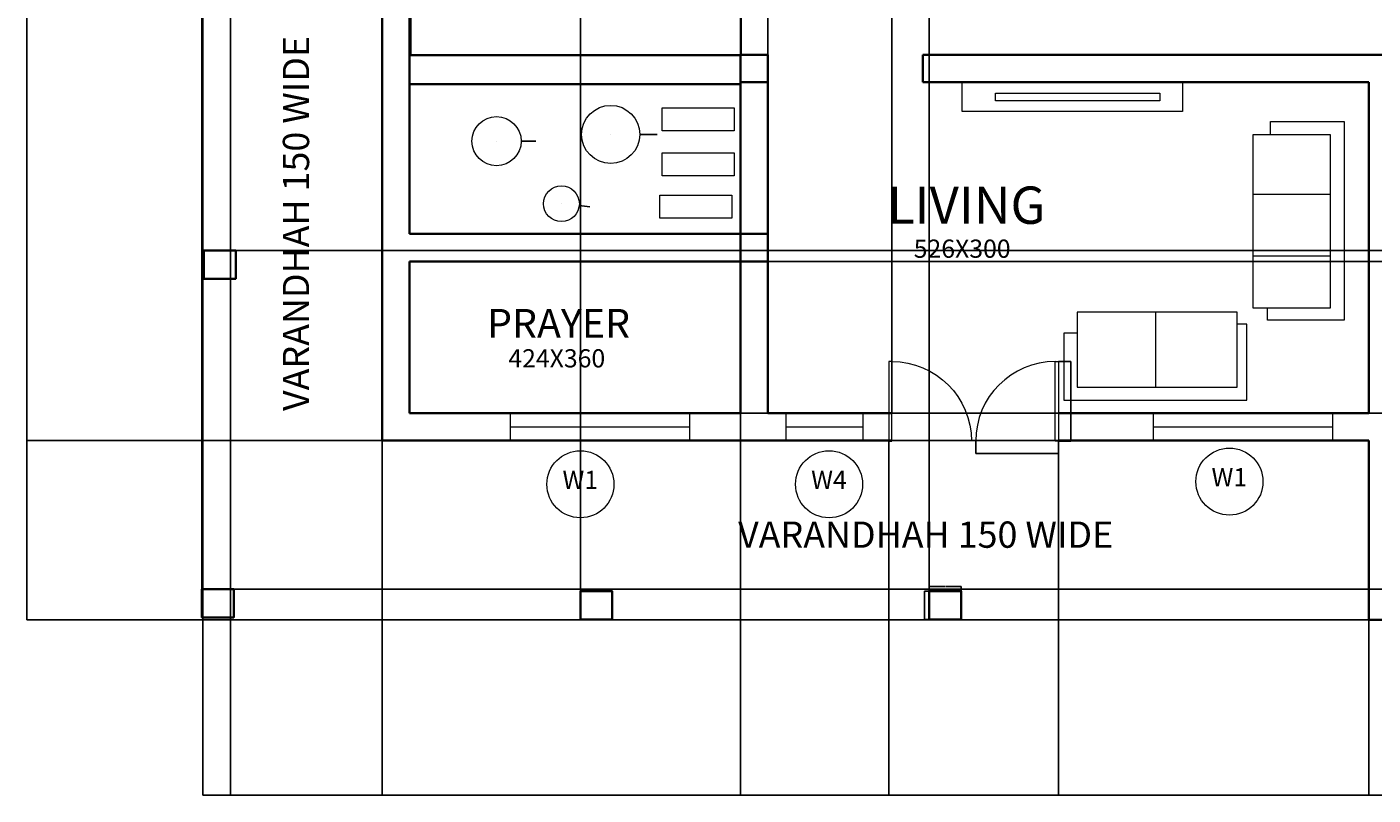
# Model space of a CAD drawing. Units: millimetres. Extents: x -2968 to 14333, y -2966 to 13411.
# Tile 1 of 3: x -2968 to 8301, y -2966 to 3466. Entities that reach past the tile are written whole.
import ezdxf

# ---------------------------------------------------------------- set-up
doc = ezdxf.new("R2010")
doc.units = ezdxf.units.MM
doc.header["$MEASUREMENT"] = 0
for name, color, linetype, lineweight in [('A-ANNO-DIMS', 2, 'Continuous', 18), ('A-ANNO-SYMB', 3, 'Continuous', 13), ('A-AREA-IDEN', 7, 'Continuous', 18), ('A-COLS', 7, 'Continuous', 35), ('A-DOOR', 3, 'Continuous', 18), ('A-FLOR-DETL', 8, 'Continuous', 18), ('A-FLOR-EDGE', 7, 'Continuous', 25), ('A-FURN', 8, 'Continuous', 18), ('A-GLAZ', 4, 'Continuous', 18), ('A-WALL', 7, 'Continuous', 35)]:
    doc.layers.add(name, color=color, linetype=linetype, lineweight=lineweight)
doc.styles.get("Standard").update_dxf_attribs({"font": 'arial.ttf'})
doc.dimstyles.get("Standard").update_dxf_attribs({"dimtxt": 0.18, "dimasz": 0.18, "dimexe": 0.18, "dimexo": 0.0625, "dimgap": 0.09, "dimtad": 0, "dimtih": 1, "dimtoh": 1, "dimdec": 4, "dimzin": 0, "dimdsep": 46, "dimtxsty": 'Standard', "dimcen": 0.09, "dimadec": 0, "dimazin": 0, "dimtfac": 1, "dimtdec": 4, "dimtofl": 0, "dimtmove": 0, "dimatfit": 3, "dimfxl": 1, "dimtolj": 1, "dimtzin": 0, "dimarcsym": 0})

# ---------------------------------------------------------------- blocks, each defined once
blk = doc.blocks.new('DOOR-SWING-666')
blk.add_lwpolyline([(666.2992070210612, -7.87249337009e-05), (666.2992070210612, 666.0645318323222), (692.9797223629398, 666.0645318323222), (692.9797223629398, -7.87249337009e-05)], close=True)
blk.add_arc((666.2992070210612, -7.87249337009e-05), 666.2995763929106, 90, 180)
blk = doc.blocks.new('WIN-1500')
for p, q in [((-0.0001454069465439, 230.0001364428754), (-0.0001454069465439, 0.0001364428753732)), ((1499.999854593053, 230.0001364428754), (1499.999854593053, 0.0001364428753732)), ((-0.0001454069465439, 115.0001364428753), (1499.999854593053, 115.0001364428753))]:
    blk.add_line(p, q)
blk = doc.blocks.new('WIN-645')
for p, q in [((-0.0001783325678844, 645.3165217330161), (229.9998216674321, 645.3165217330161)), ((114.9998216674321, 645.3165217330161), (114.9998216674321, 9.39247611313e-05)), ((-0.0001783325678844, 9.39247611313e-05), (229.9998216674321, 9.39247611313e-05))]:
    blk.add_line(p, q)
blk = doc.blocks.new('VERANDAH-POST')
blk.add_lwpolyline([(-5.84108229305e-05, 235.3216454025205), (266.2404368537072, 235.3216454025205), (266.2404368537072, -0.0003482651118247), (-5.84108229305e-05, -0.0003482651118247)], close=True)
blk = doc.blocks.new('TAG-W1')
blk.add_circle((280.793431040287, 280.7932079668344), 280.7929963504647)
blk.add_text('W1', height=152.3112078732942).set_placement((130.9915239926576, 241.6268535788358))
blk = doc.blocks.new('TAG-W4')
blk.add_circle((280.792632550478, 280.7926029835935), 280.7929963504647)
blk.add_text('W4', height=152.3112078732942).set_placement((130.9907255028486, 241.6262485955949))
blk = doc.blocks.new('*D26')
at = {"layer": 'A-ANNO-DIMS', "color": 0, "lineweight": -2, "transparency": 16777216}
for p, q in [((4974.697580339908, -2.140366612195065), (4974.697580339908, -106.2048803724133)), ((4974.877580339908, -106.0248803724133), (5319.720982278243, -106.0248803724133)), ((5667.497672074696, -106.0248803724133), (5322.654270136361, -106.0248803724133)), ((5667.677672074696, -2.140366612195065), (5667.677672074696, -106.2048803724133))]:
    blk.add_line(p, q, dxfattribs=at)
at = {"layer": 'A-ANNO-DIMS', "color": 0, "transparency": 16777216}
for points in [[(4974.877580339908, -105.9948803724133), (4974.877580339908, -106.0548803724133), (4974.697580339908, -106.0248803724133)], [(5667.497672074696, -105.9948803724133), (5667.497672074696, -106.0548803724133), (5667.677672074696, -106.0248803724133)]]:
    blk.add_solid(points, dxfattribs=at)
at = {"layer": 'Defpoints', "color": 0, "transparency": 16777216}
for p in [(4974.697580339908, -2.077866612195065), (5667.677672074696, -2.077866612195065), (5667.677672074696, -106.0248803724133)]:
    blk.add_point(p, dxfattribs=at)
at = {"layer": 'A-ANNO-DIMS', "color": 0, "transparency": 16777216, "insert": (5321.187626207302, -106.0248803724133), "char_height": 0.18, "attachment_point": 5}
blk.add_mtext('\\A1;DOOR SWING 693 TYP.', dxfattribs=at)
blk = doc.blocks.new('*D27')
at = {"layer": 'A-ANNO-DIMS', "color": 0, "lineweight": -2, "transparency": 16777216}
for p, q in [((5667.740172074698, 664.2217097807157), (5771.804685834919, 664.2217097807157)), ((5771.624685834918, 664.0417097807158), (5771.624685834918, 331.2538247220503)), ((5771.624685834918, -1.897866612195049), (5771.624685834918, 330.8900184464705)), ((5667.740172074698, -2.077866612195066), (5771.804685834919, -2.077866612195049))]:
    blk.add_line(p, q, dxfattribs=at)
at = {"layer": 'A-ANNO-DIMS', "color": 0, "transparency": 16777216}
for points in [[(5771.594685834919, 664.0417097807158), (5771.654685834918, 664.0417097807158), (5771.624685834918, 664.2217097807157)], [(5771.594685834919, -1.897866612195049), (5771.654685834918, -1.897866612195049), (5771.624685834918, -2.077866612195049)]]:
    blk.add_solid(points, dxfattribs=at)
at = {"layer": 'Defpoints', "color": 0, "transparency": 16777216}
for p in [(5667.677672074699, 664.2217097807157), (5771.624685834918, 664.2217097807157), (5667.677672074699, -2.077866612195066)]:
    blk.add_point(p, dxfattribs=at)
at = {"layer": 'A-ANNO-DIMS', "color": 0, "transparency": 16777216, "insert": (5771.624685834918, 331.0719215842587), "char_height": 0.18, "attachment_point": 5}
blk.add_mtext('\\A1;666 TYP.', dxfattribs=at)
blk = doc.blocks.new('*D30')
at = {"layer": 'A-ANNO-DIMS', "color": 0, "lineweight": -2, "transparency": 16777216}
for p, q in [((4585.778315827249, -1259.254557985812), (4585.778315827249, -1219.200983696133)), ((4585.958315827249, -1219.380983696133), (4717.185064141641, -1219.380983696133)), ((4851.838811091778, -1219.380983696133), (4720.612062777385, -1219.380983696133)), ((4852.018811091778, -1259.254557985812), (4852.018811091778, -1219.200983696133))]:
    blk.add_line(p, q, dxfattribs=at)
at = {"layer": 'A-ANNO-DIMS', "color": 0, "transparency": 16777216}
for points in [[(4585.958315827249, -1219.350983696133), (4585.958315827249, -1219.410983696133), (4585.778315827249, -1219.380983696133)], [(4851.838811091778, -1219.350983696133), (4851.838811091778, -1219.410983696133), (4852.018811091778, -1219.380983696133)]]:
    blk.add_solid(points, dxfattribs=at)
at = {"layer": 'Defpoints', "color": 0, "transparency": 16777216}
for p in [(4852.018811091778, -1219.380983696133), (4585.778315827249, -1259.317057985812), (4852.018811091778, -1259.317057985812)]:
    blk.add_point(p, dxfattribs=at)
at = {"layer": 'A-ANNO-DIMS', "color": 0, "transparency": 16777216, "insert": (4718.898563459513, -1219.380983696133), "char_height": 0.18, "attachment_point": 5}
blk.add_mtext('\\A1;VERANDAH POST 266 TYP.', dxfattribs=at)
blk = doc.blocks.new('*D31')
at = {"layer": 'A-ANNO-DIMS', "color": 0, "lineweight": -2, "transparency": 16777216}
for p, q in [((4585.71581582725, -1259.317057985813), (4545.662241537573, -1259.317057985813)), ((4545.842241537573, -1259.497057985813), (4545.842241537573, -1376.796090290297)), ((4545.842241537573, -1494.459051653445), (4545.842241537573, -1377.16001934896)), ((4585.71581582725, -1494.639051653445), (4545.662241537573, -1494.639051653445))]:
    blk.add_line(p, q, dxfattribs=at)
at = {"layer": 'A-ANNO-DIMS', "color": 0, "transparency": 16777216}
for points in [[(4545.812241537572, -1259.497057985813), (4545.872241537572, -1259.497057985813), (4545.842241537573, -1259.317057985813)], [(4545.812241537572, -1494.459051653445), (4545.872241537572, -1494.459051653445), (4545.842241537573, -1494.639051653445)]]:
    blk.add_solid(points, dxfattribs=at)
at = {"layer": 'Defpoints', "color": 0, "transparency": 16777216}
for p in [(4545.842241537573, -1259.317057985813), (4585.77831582725, -1259.317057985813), (4585.77831582725, -1494.639051653445)]:
    blk.add_point(p, dxfattribs=at)
at = {"layer": 'A-ANNO-DIMS', "color": 0, "transparency": 16777216, "insert": (4545.842241537571, -1376.97805481963), "char_height": 0.18, "attachment_point": 5}
blk.add_mtext('\\A1;235 TYP.', dxfattribs=at)
blk = doc.blocks.new('*D33')
at = {"layer": 'A-ANNO-DIMS', "color": 0, "lineweight": -2, "transparency": 16777216}
for p, q in [((-1494.873479, 11907.507473), (-2967.835419000003, 11907.507473)), ((-2967.655419000003, 11907.327473), (-2967.655419000002, 5205.189437529332)), ((-2967.655419, -1497.312527000001), (-2967.655419000002, 5204.825508470669)), ((-1494.873479, -1497.492527), (-2967.835419, -1497.492527000001))]:
    blk.add_line(p, q, dxfattribs=at)
at = {"layer": 'A-ANNO-DIMS', "color": 0, "transparency": 16777216}
for points in [[(-2967.685419000004, 11907.327473), (-2967.625419000004, 11907.327473), (-2967.655419000003, 11907.507473)], [(-2967.685419, -1497.312527000001), (-2967.625419, -1497.312527000001), (-2967.655419, -1497.492527000001)]]:
    blk.add_solid(points, dxfattribs=at)
at = {"layer": 'Defpoints', "color": 0, "transparency": 16777216}
for p in [(-2967.655419000003, 11907.507473), (-1494.810979, 11907.507473), (-1494.810979, -1497.492527)]:
    blk.add_point(p, dxfattribs=at)
at = {"layer": 'A-ANNO-DIMS', "color": 0, "transparency": 16777216, "insert": (-2967.655419, 5205.007473000001), "char_height": 0.18, "attachment_point": 5}
blk.add_mtext('\\A1;13405', dxfattribs=at)
blk = doc.blocks.new('*D34')
at = {"layer": 'A-ANNO-DIMS', "color": 0, "lineweight": -2, "transparency": 16777216}
for p, q in [((5.189021, 2.444973), (5.189020999999818, -2966.059788)), ((-1494.810979, -1497.555027), (-1494.810979, -2966.059788000001)), ((-1494.630979, -2965.879788), (-745.1609721787177, -2965.879788)), ((5.009020999999818, -2965.879788), (-744.4609858212825, -2965.879788))]:
    blk.add_line(p, q, dxfattribs=at)
at = {"layer": 'A-ANNO-DIMS', "color": 0, "transparency": 16777216}
for points in [[(-1494.630979, -2965.849788), (-1494.630979, -2965.909788000001), (-1494.810979, -2965.879788)], [(5.009020999999818, -2965.849788), (5.009020999999818, -2965.909788000001), (5.189020999999818, -2965.879788)]]:
    blk.add_solid(points, dxfattribs=at)
at = {"layer": 'Defpoints', "color": 0, "transparency": 16777216}
for p in [(5.189021, 2.507473), (-1494.810979, -1497.492527), (5.189020999999818, -2965.879788)]:
    blk.add_point(p, dxfattribs=at)
at = {"layer": 'A-ANNO-DIMS', "color": 0, "transparency": 16777216, "insert": (-744.8109790000001, -2965.879788), "char_height": 0.18, "attachment_point": 5}
blk.add_mtext('\\A1;1500', dxfattribs=at)
blk = doc.blocks.new('*D35')
at = {"layer": 'A-ANNO-DIMS', "color": 0, "lineweight": -2, "transparency": 16777216}
for p, q in [((5.189021, 2.444973), (5.189020999999818, -2966.059788)), ((8265.189021, -1497.555027), (8265.189021, -2966.059788000001)), ((5.369020999999817, -2965.879788), (4134.830433005457, -2965.879788)), ((8265.009021, -2965.879788), (4135.547608994543, -2965.879788))]:
    blk.add_line(p, q, dxfattribs=at)
at = {"layer": 'A-ANNO-DIMS', "color": 0, "transparency": 16777216}
for points in [[(5.369020999999817, -2965.849788), (5.369020999999817, -2965.909788000001), (5.189020999999818, -2965.879788)], [(8265.009021, -2965.849788), (8265.009021, -2965.909788000001), (8265.189021, -2965.879788)]]:
    blk.add_solid(points, dxfattribs=at)
at = {"layer": 'Defpoints', "color": 0, "transparency": 16777216}
for p in [(5.189021, 2.507473), (8265.189021, -1497.492527), (8265.189021, -2965.879788)]:
    blk.add_point(p, dxfattribs=at)
at = {"layer": 'A-ANNO-DIMS', "color": 0, "transparency": 16777216, "insert": (4135.189021, -2965.879788), "char_height": 0.18, "attachment_point": 5}
blk.add_mtext('\\A1;8260', dxfattribs=at)
blk = doc.blocks.new('*D36')
at = {"layer": 'A-ANNO-DIMS', "color": 0, "lineweight": -2, "transparency": 16777216}
for p, q in [((8265.189021, -1497.555027), (8265.189021, -2966.059788000001)), ((12815.189021, -1497.555027), (12815.189021, -2966.059788000001)), ((8265.369021, -2965.879788), (10539.82693368758, -2965.879788)), ((12815.009021, -2965.879788), (10540.55110831241, -2965.879788))]:
    blk.add_line(p, q, dxfattribs=at)
at = {"layer": 'A-ANNO-DIMS', "color": 0, "transparency": 16777216}
for points in [[(8265.369021, -2965.849788), (8265.369021, -2965.909788000001), (8265.189021, -2965.879788)], [(12815.009021, -2965.849788), (12815.009021, -2965.909788000001), (12815.189021, -2965.879788)]]:
    blk.add_solid(points, dxfattribs=at)
at = {"layer": 'Defpoints', "color": 0, "transparency": 16777216}
for p in [(8265.189021, -1497.492527), (12815.189021, -1497.492527), (12815.189021, -2965.879788)]:
    blk.add_point(p, dxfattribs=at)
at = {"layer": 'A-ANNO-DIMS', "color": 0, "transparency": 16777216, "insert": (10540.189021, -2965.879788), "char_height": 0.18, "attachment_point": 5}
blk.add_mtext('\\A1;4550', dxfattribs=at)
blk = doc.blocks.new('*D42')
at = {"layer": 'A-ANNO-DIMS', "color": 0, "lineweight": -2, "transparency": 16777216}
for p, q in [((8265.126521000004, 2.507473), (-2967.835419000003, 2.507472999998194)), ((-2967.655419000002, 2.327472999998194), (-2967.655419000002, -747.310623862212)), ((-2967.655419000001, -1497.312527000002), (-2967.655419000002, -747.674430137792)), ((8265.126521000004, -1497.492527), (-2967.835419000003, -1497.492527000002))]:
    blk.add_line(p, q, dxfattribs=at)
at = {"layer": 'A-ANNO-DIMS', "color": 0, "transparency": 16777216}
for points in [[(-2967.685419000002, 2.327472999998194), (-2967.625419000002, 2.327472999998194), (-2967.655419000002, 2.507472999998194)], [(-2967.685419000002, -1497.312527000002), (-2967.625419000001, -1497.312527000002), (-2967.655419000001, -1497.492527000002)]]:
    blk.add_solid(points, dxfattribs=at)
at = {"layer": 'Defpoints', "color": 0, "transparency": 16777216}
for p in [(-2967.655419000002, 2.507472999998194), (8265.189021000002, 2.507473), (8265.189021000002, -1497.492527)]:
    blk.add_point(p, dxfattribs=at)
at = {"layer": 'A-ANNO-DIMS', "color": 0, "transparency": 16777216, "insert": (-2967.655419000001, -747.492527000001), "char_height": 0.18, "attachment_point": 5}
blk.add_mtext('\\A1;1500', dxfattribs=at)
blk = doc.blocks.new('*D46')
at = {"layer": 'A-ANNO-DIMS', "color": 0, "lineweight": -2, "transparency": 16777216}
for p, q in [((-1264.810979, 11677.444973), (-1264.810979000001, -2966.059788000001)), ((3005.189021, 11677.444973), (3005.189021, -2966.059788000001)), ((-1264.630979000001, -2965.879788), (869.8269336875846, -2965.879788)), ((3005.009020999999, -2965.879788), (870.551108312414, -2965.879788))]:
    blk.add_line(p, q, dxfattribs=at)
at = {"layer": 'A-ANNO-DIMS', "color": 0, "transparency": 16777216}
for points in [[(-1264.630979000001, -2965.849788), (-1264.630979000001, -2965.909788000001), (-1264.810979000001, -2965.879788)], [(3005.009020999999, -2965.849788), (3005.009020999999, -2965.909788000001), (3005.189021, -2965.879788)]]:
    blk.add_solid(points, dxfattribs=at)
at = {"layer": 'Defpoints', "color": 0, "transparency": 16777216}
for p in [(-1264.810979, 11677.507473), (3005.189021, 11677.507473), (3005.189021, -2965.879788)]:
    blk.add_point(p, dxfattribs=at)
at = {"layer": 'A-ANNO-DIMS', "color": 0, "transparency": 16777216, "insert": (870.1890209999993, -2965.879788), "char_height": 0.18, "attachment_point": 5}
blk.add_mtext('\\A1;4270', dxfattribs=at)
blk = doc.blocks.new('*D48')
at = {"layer": 'A-ANNO-DIMS', "color": 0, "lineweight": -2, "transparency": 16777216}
for p, q in [((4246.640455, -2.140366999999999), (4246.640455, -2966.059788)), ((5667.677671999999, -2.140366999999999), (5667.677671999999, -2966.059788)), ((4246.820455, -2965.879788), (4956.826137169849, -2965.879788)), ((5667.497671999999, -2965.879788), (4957.491989830149, -2965.879788))]:
    blk.add_line(p, q, dxfattribs=at)
at = {"layer": 'A-ANNO-DIMS', "color": 0, "transparency": 16777216}
for points in [[(4246.820455, -2965.849788), (4246.820455, -2965.909788000001), (4246.640455, -2965.879788)], [(5667.497671999999, -2965.849788), (5667.497671999999, -2965.909788000001), (5667.677671999999, -2965.879788)]]:
    blk.add_solid(points, dxfattribs=at)
at = {"layer": 'Defpoints', "color": 0, "transparency": 16777216}
for p in [(4246.640455, -2.077866999999999), (5667.677671999999, -2.077866999999999), (5667.677671999999, -2965.879788)]:
    blk.add_point(p, dxfattribs=at)
at = {"layer": 'A-ANNO-DIMS', "color": 0, "transparency": 16777216, "insert": (4957.159063499999, -2965.879788), "char_height": 0.18, "attachment_point": 5}
blk.add_mtext('\\A1;1421', dxfattribs=at)
blk = doc.blocks.new('*D49')
at = {"layer": 'A-ANNO-DIMS', "color": 0, "lineweight": -2, "transparency": 16777216}
for p, q in [((3235.189021, 232.569973), (3235.189021000001, 13410.507299)), ((3235.369021000001, 13410.327299), (3753.817212416781, 13410.327299)), ((4273.14097, 13410.327299), (3754.69277858322, 13410.327299)), ((4273.320969999999, 232.569973), (4273.320970000001, 13410.507299))]:
    blk.add_line(p, q, dxfattribs=at)
at = {"layer": 'A-ANNO-DIMS', "color": 0, "transparency": 16777216}
for points in [[(3235.369021000001, 13410.357299), (3235.369021000001, 13410.297299), (3235.189021000001, 13410.327299)], [(4273.14097, 13410.357299), (4273.14097, 13410.297299), (4273.320970000001, 13410.327299)]]:
    blk.add_solid(points, dxfattribs=at)
at = {"layer": 'Defpoints', "color": 0, "transparency": 16777216}
for p in [(4273.320970000001, 13410.327299), (3235.189021, 232.507473), (4273.320969999999, 232.507473)]:
    blk.add_point(p, dxfattribs=at)
at = {"layer": 'A-ANNO-DIMS', "color": 0, "transparency": 16777216, "insert": (3754.254995500001, 13410.327299), "char_height": 0.18, "attachment_point": 5}
blk.add_mtext('\\A1;1038.1', dxfattribs=at)
blk = doc.blocks.new('*D53')
at = {"layer": 'A-ANNO-DIMS', "color": 0, "lineweight": -2, "transparency": 16777216}
for p, q in [((-1220.345468, 1592.680140000001), (14333.28935600001, 1592.680140000003)), ((14333.10935600001, 1592.500140000003), (14333.10935600001, 175.1113265293341)), ((14333.10935600001, -1242.641415999998), (14333.10935600001, 174.7473974706711)), ((-1236.815201, -1242.821416), (14333.28935600001, -1242.821415999998))]:
    blk.add_line(p, q, dxfattribs=at)
at = {"layer": 'A-ANNO-DIMS', "color": 0, "transparency": 16777216}
for points in [[(14333.07935600001, 1592.500140000003), (14333.13935600001, 1592.500140000003), (14333.10935600001, 1592.680140000003)], [(14333.07935600001, -1242.641415999998), (14333.13935600001, -1242.641415999998), (14333.10935600001, -1242.821415999998)]]:
    blk.add_solid(points, dxfattribs=at)
at = {"layer": 'Defpoints', "color": 0, "transparency": 16777216}
for p in [(-1220.407968, 1592.680140000001), (14333.10935600001, 1592.680140000003), (-1236.877701, -1242.821416)]:
    blk.add_point(p, dxfattribs=at)
at = {"layer": 'A-ANNO-DIMS', "color": 0, "transparency": 16777216, "insert": (14333.10935600001, 174.9293619999985), "char_height": 0.18, "attachment_point": 5}
blk.add_mtext('\\A1;2835.5', dxfattribs=at)
blk = doc.blocks.new('*D54')
at = {"layer": 'A-ANNO-DIMS', "color": 0, "lineweight": -2, "transparency": 16777216}
for p, q in [((-1220.345468, 3884.149375000002), (14333.28935600001, 3884.149375000005)), ((14333.10935600001, 3883.969375000005), (14333.10935600001, 2738.596660637794)), ((14333.10935600001, 1592.860140000003), (14333.10935600001, 2738.232854362214)), ((-1220.345468, 1592.680140000001), (14333.28935600001, 1592.680140000003))]:
    blk.add_line(p, q, dxfattribs=at)
at = {"layer": 'A-ANNO-DIMS', "color": 0, "transparency": 16777216}
for points in [[(14333.07935600001, 3883.969375000005), (14333.13935600001, 3883.969375000005), (14333.10935600001, 3884.149375000005)], [(14333.07935600001, 1592.860140000003), (14333.13935600001, 1592.860140000003), (14333.10935600001, 1592.680140000003)]]:
    blk.add_solid(points, dxfattribs=at)
at = {"layer": 'Defpoints', "color": 0, "transparency": 16777216}
for p in [(-1220.407968, 3884.149375000002), (14333.10935600001, 3884.149375000005), (-1220.407968, 1592.680140000001)]:
    blk.add_point(p, dxfattribs=at)
at = {"layer": 'A-ANNO-DIMS', "color": 0, "transparency": 16777216, "insert": (14333.10935600001, 2738.414757499999), "char_height": 0.18, "attachment_point": 5}
blk.add_mtext('\\A1;2291.5', dxfattribs=at)
blk = doc.blocks.new('*D56')
at = {"layer": 'A-ANNO-DIMS', "color": 0, "lineweight": -2, "transparency": 16777216}
for p, q in [((-1503.118196, -1242.758916), (-1503.118195999999, 13410.507299)), ((-1502.938195999999, 13410.327299), (80.61449804775, 13410.327299)), ((1664.884982000001, 13410.327299), (81.33228795225203, 13410.327299)), ((1665.064982, -1259.254558), (1665.064982000001, 13410.507299))]:
    blk.add_line(p, q, dxfattribs=at)
at = {"layer": 'A-ANNO-DIMS', "color": 0, "transparency": 16777216}
for points in [[(-1502.938195999999, 13410.357299), (-1502.938195999999, 13410.297299), (-1503.118195999999, 13410.327299)], [(1664.884982000001, 13410.357299), (1664.884982000001, 13410.297299), (1665.064982000001, 13410.327299)]]:
    blk.add_solid(points, dxfattribs=at)
at = {"layer": 'Defpoints', "color": 0, "transparency": 16777216}
for p in [(1665.064982000001, 13410.327299), (-1503.118196, -1242.821416), (1665.064982, -1259.317058)]:
    blk.add_point(p, dxfattribs=at)
at = {"layer": 'A-ANNO-DIMS', "color": 0, "transparency": 16777216, "insert": (80.97339300000101, 13410.327299), "char_height": 0.18, "attachment_point": 5}
blk.add_mtext('\\A1;3168', dxfattribs=at)
blk = doc.blocks.new('*D57')
at = {"layer": 'A-ANNO-DIMS', "color": 0, "lineweight": -2, "transparency": 16777216}
for p, q in [((1665.064982, -1259.254558), (1665.064982000001, 13410.507299)), ((1665.244982000001, 13410.327299), (3125.078715848568, 13410.327299)), ((4585.598316000001, 13410.327299), (3125.764582151433, 13410.327299)), ((4585.778315999999, -1259.254558), (4585.778316000001, 13410.507299))]:
    blk.add_line(p, q, dxfattribs=at)
at = {"layer": 'A-ANNO-DIMS', "color": 0, "transparency": 16777216}
for points in [[(1665.244982000001, 13410.357299), (1665.244982000001, 13410.297299), (1665.064982000001, 13410.327299)], [(4585.598316000001, 13410.357299), (4585.598316000001, 13410.297299), (4585.778316000001, 13410.327299)]]:
    blk.add_solid(points, dxfattribs=at)
at = {"layer": 'Defpoints', "color": 0, "transparency": 16777216}
for p in [(4585.778316000001, 13410.327299), (1665.064982, -1259.317058), (4585.778315999999, -1259.317058)]:
    blk.add_point(p, dxfattribs=at)
at = {"layer": 'A-ANNO-DIMS', "color": 0, "transparency": 16777216, "insert": (3125.421649000001, 13410.327299), "char_height": 0.18, "attachment_point": 5}
blk.add_mtext('\\A1;2921', dxfattribs=at)
blk = doc.blocks.new('*D58')
at = {"layer": 'A-ANNO-DIMS', "color": 0, "lineweight": -2, "transparency": 16777216}
for p, q in [((244.489985, 3229.006698), (244.4899850000006, 13410.507299)), ((244.6699850000006, 13410.327299), (1627.163433433834, 13410.327299)), ((3010.377373000001, 13410.327299), (1627.883924566167, 13410.327299)), ((3010.557373000001, 3229.006698), (3010.557373000001, 13410.507299))]:
    blk.add_line(p, q, dxfattribs=at)
at = {"layer": 'A-ANNO-DIMS', "color": 0, "transparency": 16777216}
for points in [[(244.6699850000006, 13410.357299), (244.6699850000006, 13410.297299), (244.4899850000006, 13410.327299)], [(3010.377373000001, 13410.357299), (3010.377373000001, 13410.297299), (3010.557373000001, 13410.327299)]]:
    blk.add_solid(points, dxfattribs=at)
at = {"layer": 'Defpoints', "color": 0, "transparency": 16777216}
for p in [(3010.557373000001, 13410.327299), (244.489985, 3228.944198), (3010.557373000001, 3228.944198)]:
    blk.add_point(p, dxfattribs=at)
at = {"layer": 'A-ANNO-DIMS', "color": 0, "transparency": 16777216, "insert": (1627.523679, 13410.327299), "char_height": 0.18, "attachment_point": 5}
blk.add_mtext('\\A1;2766', dxfattribs=at)
blk = doc.blocks.new('*D62')
at = {"layer": 'A-ANNO-DIMS', "color": 0, "lineweight": -2, "transparency": 16777216}
for p, q in [((235.2515210000001, 1502.507473), (14333.28935600001, 1502.507473000003)), ((14333.10935600001, 1502.327473000002), (14333.10935600001, 867.6893761377925)), ((14333.10935600001, 232.6874730000024), (14333.10935600001, 867.3255698622125)), ((235.2515210000001, 232.5074730000001), (14333.28935600001, 232.5074730000024))]:
    blk.add_line(p, q, dxfattribs=at)
at = {"layer": 'A-ANNO-DIMS', "color": 0, "transparency": 16777216}
for points in [[(14333.07935600001, 1502.327473000002), (14333.13935600001, 1502.327473000002), (14333.10935600001, 1502.507473000003)], [(14333.07935600001, 232.6874730000024), (14333.13935600001, 232.6874730000024), (14333.10935600001, 232.5074730000024)]]:
    blk.add_solid(points, dxfattribs=at)
at = {"layer": 'Defpoints', "color": 0, "transparency": 16777216}
for p in [(235.1890210000001, 1502.507473), (14333.10935600001, 1502.507473000003), (235.1890210000001, 232.5074730000001)]:
    blk.add_point(p, dxfattribs=at)
at = {"layer": 'A-ANNO-DIMS', "color": 0, "transparency": 16777216, "insert": (14333.10935600001, 867.5074729999982), "char_height": 0.18, "attachment_point": 5}
blk.add_mtext('\\A1;1270', dxfattribs=at)
blk = doc.blocks.new('*D68')
at = {"layer": 'A-ANNO-DIMS', "color": 0, "lineweight": -2, "transparency": 16777216}
for p, q in [((1918.923728, 2565.707111999999), (1919.103728, 2565.707111999999)), ((1919.013728, 2565.617111999999), (1919.013728, 2565.797111999999)), ((2308.276335999984, 2565.706932799999), (2162.482857999999, 2565.706999917135))]:
    blk.add_line(p, q, dxfattribs=at)
at = {"layer": 'A-ANNO-DIMS', "color": 0, "transparency": 16777216}
blk.add_solid([(2162.48285801381, 2565.736999917135), (2162.482857986188, 2565.676999917135), (2162.302857999999, 2565.706999999999)], dxfattribs=at)
at = {"layer": 'Defpoints', "color": 0, "transparency": 16777216}
for p in [(1675.724597999999, 2565.707224), (2162.302857999999, 2565.706999999999)]:
    blk.add_point(p, dxfattribs=at)
at = {"layer": 'A-ANNO-DIMS', "color": 0, "transparency": 16777216, "insert": (2308.767898073654, 2565.706932799999), "char_height": 0.18, "attachment_point": 5}
blk.add_mtext('\\A1;∅486.6', dxfattribs=at)
blk = doc.blocks.new('*D69')
at = {"layer": 'A-ANNO-DIMS', "color": 0, "lineweight": -2, "transparency": 16777216}
for p, q in [((963.5581299999998, 2509.548519000001), (963.7381300000001, 2509.548519000001)), ((963.6481299999999, 2509.458519), (963.6481299999999, 2509.638519000001)), ((1293.042784399662, 2509.549288600001), (1169.699788999999, 2509.549000420554))]:
    blk.add_line(p, q, dxfattribs=at)
at = {"layer": 'A-ANNO-DIMS', "color": 0, "transparency": 16777216}
blk.add_solid([(1169.699788929907, 2509.579000420555), (1169.699789070092, 2509.519000420554), (1169.519789, 2509.549000000001)], dxfattribs=at)
at = {"layer": 'Defpoints', "color": 0, "transparency": 16777216}
for p in [(757.7764709999999, 2509.548038000001), (1169.519789, 2509.549000000001)]:
    blk.add_point(p, dxfattribs=at)
at = {"layer": 'A-ANNO-DIMS', "color": 0, "transparency": 16777216, "insert": (1293.603964481518, 2509.549288600001), "char_height": 0.18, "attachment_point": 5}
blk.add_mtext('\\A1;∅411.74', dxfattribs=at)
blk = doc.blocks.new('*D70')
at = {"layer": 'A-ANNO-DIMS', "color": 0, "lineweight": -2, "transparency": 16777216}
for p, q in [((1506.817108, 1985.509606999999), (1506.997108, 1985.509606999999)), ((1506.907108, 1985.419607), (1506.907108, 1985.599606999999)), ((1745.161788065114, 1960.387819793133), (1655.995290666339, 1969.789615271071))]:
    blk.add_line(p, q, dxfattribs=at)
at = {"layer": 'A-ANNO-DIMS', "color": 0, "transparency": 16777216}
blk.add_solid([(1655.998436454493, 1969.819449882127), (1655.992144878184, 1969.759780660014), (1655.816283, 1969.808489999999)], dxfattribs=at)
at = {"layer": 'Defpoints', "color": 0, "transparency": 16777216}
for p in [(1357.997933, 2001.210724), (1655.816283, 1969.808489999999)]:
    blk.add_point(p, dxfattribs=at)
at = {"layer": 'A-ANNO-DIMS', "color": 0, "transparency": 16777216, "insert": (1745.723336496219, 1960.387819793133), "char_height": 0.18, "attachment_point": 5}
blk.add_mtext('\\A1;∅299.47', dxfattribs=at)

msp = doc.modelspace()

# ---------------------------------------------------------------- linework, layer by layer
at = {"layer": 'A-FLOR-DETL'}
for points in [[(2349.224944576621, 2788.2255512923), (2952.610556416214, 2788.2255512923), (2952.610556416214, 2594.963126730174), (2349.224944576621, 2594.963126730174)], [(2349.224944576621, 2410.898534014821), (2952.610556416214, 2410.898534014821), (2952.610556416214, 2217.636109452695), (2349.224944576621, 2217.636109452695)], [(2330.817596264184, 2056.566096354276), (2934.203208103776, 2056.566096354276), (2934.203208103776, 1863.303671792149), (2330.817596264184, 1863.303671792149)]]:
    msp.add_lwpolyline(points, close=True, dxfattribs=at)
for centre, radius in [((963.6481301560998, 2509.54851924628), 205.8716588318348), ((1919.013728111982, 2565.70711228624), 243.2891297005117), ((1506.907107524574, 1985.509606663137), 149.7346569485962)]:
    msp.add_circle(centre, radius, dxfattribs=at)
at = {"layer": 'A-FLOR-EDGE'}
for p, q in [((-1494.810978557335, 2.507473364634584), (-1494.810978557335, 6657.507473364635)), ((-1494.810978557335, 2.507473364634584), (-1494.810978557335, -1497.492526635365)), ((8265.189021442662, -1497.492526635365), (-1494.810978557336, -1497.492526635365))]:
    msp.add_line(p, q, dxfattribs=at)
at = {"layer": 'A-FURN'}
for p, q in [((7297.897933750181, 2064.55783755082), (7942.255744674709, 2064.55783755082)), ((6478.718142271041, 1078.002830510144), (6478.718142271041, 450.4752302423002))]:
    msp.add_line(p, q, dxfattribs=at)
for points in [[(4862.181595582515, 3001.579722309194), (6705.869539797307, 3001.579722309194), (6705.869539797307, 2757.382163017465), (4862.181595582515, 2757.382163017465)], [(5141.527579856338, 2910.878040781419), (6517.310166411101, 2910.878040781419), (6517.310166411101, 2848.084340193658), (5141.527579856338, 2848.084340193658)], [(7298.680505050812, 2564.81431889988), (7940.786512232851, 2564.81431889988), (7940.786512232851, 1110.145631702966), (7298.680505050812, 1110.145631702966)], [(7162.26289832429, 1078.002830510144), (5822.885862275725, 1078.002830510144), (5822.885862275725, 450.4752302423002), (7162.26289832429, 450.4752302423002)]]:
    msp.add_lwpolyline(points, close=True, dxfattribs=at)
for points in [[(7443.381135543808, 2564.81431889988), (7443.381135543808, 2673.236423376715), (8058.355687633158, 2673.236423376715), (8058.355687633158, 1010.75870259921), (7416.249680451118, 1010.75870259921), (7416.249680451118, 1110.145631702966)], [(7297.897933750181, 1550.277974950382), (7938.655638691503, 1550.277974950382)], [(5822.885862275725, 902.6642217397457), (5712.041518052108, 902.6642217397457), (5712.041518052108, 339.7349780217628), (7245.396156492176, 339.7349780217628), (7245.396156492176, 976.4910565534373), (7162.26289832429, 976.4910565534373)]]:
    msp.add_lwpolyline(points, dxfattribs=at)
at = {"layer": 'A-WALL'}
for p, q in [((5.189021442664909, 2.507473364634584), (5.189021442664909, 6887.507473364634)), ((235.1890214426649, 1732.507473364634), (235.1890214426649, 6657.507473364635)), ((3010.557373329997, 3228.944198388607), (244.489985473454, 3228.944198388607)), ((3005.189021442665, 232.5074733646347), (3005.189021442665, 3232.507473364635)), ((3005.189021442665, 3232.507473364635), (3235.189021442665, 3232.507473364635)), ((3235.189021442665, 232.5074733646346), (3235.189021442665, 3232.507473364635)), ((4530.982965129427, 3002.507473364635), (4530.982965129427, 3232.507473364635)), ((4530.982965129427, 3232.507473364635), (8495.189021442664, 3232.507473364635)), ((3003.291314780712, 2987.684637214989), (237.1633764356375, 2987.684637214989)), ((3005.189021442665, 3002.507473364635), (3235.189021442665, 3002.507473364635)), ((4530.982965129426, 3002.507473364635), (8265.189021442666, 3002.507473364635)), ((8265.189021442662, 232.5074733646346), (8265.189021442666, 3002.507473364635)), ((235.1890214426649, 1732.507473364634), (3235.189021442665, 1732.507473364634)), ((235.1890214426649, 232.5074733646346), (235.1890214426649, 1502.507473364634)), ((235.1890214426649, 1502.507473364634), (3235.189021442665, 1502.507473364634)), ((235.1890214426649, 232.5074733646346), (3005.189021442665, 232.5074733646346)), ((3235.189021442665, 232.5074733646346), (4273.320970137967, 232.5074733646346)), ((5667.677672074696, 232.5074733646346), (8265.189021442662, 232.5074733646346)), ((5.189021442664909, 2.507473364634584), (4273.320970137967, 2.507473364634584)), ((5667.677672074696, 2.507473364634584), (8265.189021442662, 2.507473364634584)), ((8265.189021442662, 2.507473364634584), (8265.189021442662, -1497.492526635365)), ((8265.189021442662, -1497.492526635365), (12815.18902144266, -1497.492526635365))]:
    msp.add_line(p, q, dxfattribs=at)

# ---------------------------------------------------------------- block references
at = {"layer": 'A-ANNO-SYMB'}
for name, p in [('TAG-W1', (1384.695404272141, -644.5307655195851)), ('TAG-W4', (3466.119224033774, -644.5301605363502)), ('TAG-W1', (6817.830132286608, -622.2918763133848))]:
    msp.add_blockref(name, p, dxfattribs=at)
at = {"layer": 'A-COLS'}
for p in [(-1486.648404935241, 1357.358495003373), (-1503.118137644471, -1478.143061296254), (1665.065040303527, -1494.638703388331), (4585.778374238072, -1494.638703388333)]:
    msp.add_blockref('VERANDAH-POST', p, dxfattribs=at)
at = {"layer": 'A-DOOR', "extrusion": (0, 0, -1), "zscale": -1}
msp.add_blockref('DOOR-SWING-666', (-4939.620177159028, -2.077787887259546), dxfattribs=at)
at = {"layer": 'A-DOOR'}
msp.add_blockref('DOOR-SWING-666', (4974.697949711757, -2.077787887261365), dxfattribs=at)
at = {"layer": 'A-GLAZ'}
for p in [(1078.375832292736, 2.998437439053304), (6460.65520765704, 2.749126274857189)]:
    msp.add_blockref('WIN-1500', p, dxfattribs=at)
at = {"layer": 'A-GLAZ', "rotation": 90.00000000000006}
msp.add_blockref('WIN-645', (4033.445622674138, 1.846141907519267), dxfattribs=at)

# ---------------------------------------------------------------- texts
at = {"layer": 'A-AREA-IDEN'}
msp.add_text('VARANDHAH 150 WIDE', height=220.0202070326772, rotation=90, dxfattribs=at).set_placement((-605.6366555738313, 250.0914403402658))
for s, height, p in [('LIVING', 312.237810899975, (4232.212470895338, 1817.148556295995)), ('526X300', 152.3112078732942, (4455.65262845843, 1532.937555872196)), ('PRAYER', 241.7589680836474, (883.7564674198874, 862.6084901812719)), ('424X360', 152.3112078732942, (1062.100534580042, 614.7952989119239)), ('VARANDHAH 150 WIDE', 220.0202070326772, (2985.353223411128, -895.340663461848))]:
    msp.add_text(s, height=height, dxfattribs=at).set_placement(p)

# ---------------------------------------------------------------- dimensions: what is measured, and where the dimension line sits
at = {"layer": 'A-ANNO-DIMS'}
for base, p1, p2, override, picture, middle in [((1665.064982000001, 13410.327299), (-1503.118196, -1242.821416), (1665.064982, -1259.317058), {"dimdec": 0, "dimlfac": 1, "dimrnd": 0, "dimzin": 0, "dimdsep": 46, "dimlunit": 2}, '*D56', (80.97339300000101, 13410.327299)), ((3010.557373000001, 13410.327299), (244.489985, 3228.944198), (3010.557373000001, 3228.944198), {"dimdec": 0, "dimlfac": 1, "dimrnd": 0, "dimzin": 0, "dimdsep": 46, "dimlunit": 2}, '*D58', (1627.523679, 13410.327299)), ((4585.778316000001, 13410.327299), (1665.064982, -1259.317058), (4585.778315999999, -1259.317058), {"dimdec": 0, "dimlfac": 1, "dimrnd": 0, "dimzin": 0, "dimdsep": 46, "dimlunit": 2}, '*D57', (3125.421649000001, 13410.327299)), ((4273.320970000001, 13410.327299), (3235.189021, 232.507473), (4273.320969999999, 232.507473), {"dimdec": 1, "dimlfac": 1, "dimrnd": 0, "dimzin": 0, "dimdsep": 46, "dimlunit": 2}, '*D49', (3754.254995500001, 13410.327299)), ((3005.189021, -2965.879788), (-1264.810979, 11677.507473), (3005.189021, 11677.507473), {"dimdec": 0, "dimlfac": 1, "dimrnd": 0, "dimzin": 0, "dimdsep": 46, "dimlunit": 2}, '*D46', (870.1890209999993, -2965.879788)), ((5.189020999999818, -2965.879788), (-1494.810979, -1497.492527), (5.189021, 2.507473), {"dimdec": 0, "dimlfac": 1, "dimrnd": 0, "dimzin": 0, "dimdsep": 46, "dimlunit": 2}, '*D34', (-744.8109790000001, -2965.879788)), ((8265.189021, -2965.879788), (5.189021, 2.507473), (8265.189021, -1497.492527), {"dimdec": 0, "dimlfac": 1, "dimrnd": 0, "dimzin": 0, "dimdsep": 46, "dimlunit": 2}, '*D35', (4135.189021, -2965.879788)), ((5667.677671999999, -2965.879788), (4246.640455, -2.077866999999999), (5667.677671999999, -2.077866999999999), {"dimdec": 0, "dimlfac": 1, "dimrnd": 0, "dimzin": 0, "dimdsep": 46, "dimlunit": 2}, '*D48', (4957.159063499999, -2965.879788)), ((12815.189021, -2965.879788), (8265.189021, -1497.492527), (12815.189021, -1497.492527), {"dimdec": 0, "dimlfac": 1, "dimrnd": 0, "dimzin": 0, "dimdsep": 46, "dimlunit": 2}, '*D36', (10540.189021, -2965.879788))]:
    dim = msp.add_linear_dim(base=base, p1=p1, p2=p2, dimstyle='Standard', override=override, dxfattribs=at)
    dim.commit()
    dim.dimension.update_dxf_attribs({"geometry": picture, "text_midpoint": middle})
for base, p1, p2, override, picture, middle in [((-2967.655419000003, 11907.507473), (-1494.810979, -1497.492527), (-1494.810979, 11907.507473), {"dimdec": 0, "dimlfac": 1, "dimrnd": 0, "dimzin": 0, "dimdsep": 46, "dimlunit": 2}, '*D33', (-2967.655419, 5205.007473000001)), ((14333.10935600001, 3884.149375000005), (-1220.407968, 1592.68014), (-1220.407968, 3884.149375), {"dimdec": 1, "dimlfac": 1, "dimrnd": 0, "dimzin": 0, "dimdsep": 46, "dimlunit": 2}, '*D54', (14333.10935600001, 2738.414757499999)), ((14333.10935600001, 1592.680140000003), (-1236.877701, -1242.821416), (-1220.407968, 1592.68014), {"dimdec": 1, "dimlfac": 1, "dimrnd": 0, "dimzin": 0, "dimdsep": 46, "dimlunit": 2}, '*D53', (14333.10935600001, 174.9293619999985)), ((14333.10935600001, 1502.507473000003), (235.189021, 232.507473), (235.189021, 1502.507473), {"dimdec": 0, "dimlfac": 1, "dimrnd": 0, "dimzin": 0, "dimdsep": 46, "dimlunit": 2}, '*D62', (14333.10935600001, 867.5074729999982)), ((-2967.655419000002, 2.507472999998194), (8265.189021, -1497.492527), (8265.189021, 2.507473), {"dimdec": 0, "dimlfac": 1, "dimrnd": 0, "dimzin": 0, "dimdsep": 46, "dimlunit": 2}, '*D42', (-2967.655419000001, -747.492527000001))]:
    dim = msp.add_linear_dim(base=base, p1=p1, p2=p2, angle=90, dimstyle='Standard', override=override, dxfattribs=at)
    dim.commit()
    dim.dimension.update_dxf_attribs({"geometry": picture, "text_midpoint": middle})
for p1, p2, override, picture, middle in [((757.7764709999999, 2509.548038000001), (1169.519789, 2509.549000000001), {"dimdec": 2, "dimlfac": 1, "dimrnd": 0, "dimzin": 0, "dimdsep": 46, "dimlunit": 2}, '*D69', (1293.042784399662, 2509.549288600001)), ((1675.724597999999, 2565.707224), (2162.302857999999, 2565.706999999999), {"dimdec": 1, "dimlfac": 1, "dimrnd": 0, "dimzin": 0, "dimdsep": 46, "dimlunit": 2}, '*D68', (2308.276335999984, 2565.706932799999)), ((1357.997933, 2001.210724), (1655.816283, 1969.808489999999), {"dimdec": 2, "dimlfac": 1, "dimrnd": 0, "dimzin": 0, "dimdsep": 46, "dimlunit": 2}, '*D70', (1745.161788065114, 1960.387819793133))]:
    dim = msp.add_diameter_dim_2p(p1=p1, p2=p2, dimstyle='Standard', override=override, dxfattribs=at)
    dim.commit()
    dim.dimension.update_dxf_attribs({"geometry": picture, "text_midpoint": middle, "dimtype": 163})
for base, p1, p2, picture, middle in [((5771.624685834918, 664.2217097807157), (5667.677672074696, -2.077866612195065), (5667.677672074696, 664.2217097807154), '*D27', (5771.624685834918, 331.0719215842587)), ((4545.842241537573, -1259.317057985813), (4585.778315827249, -1494.639051653445), (4585.778315827249, -1259.317057985812), '*D31', (4545.842241537571, -1376.97805481963))]:
    dim = msp.add_linear_dim(base=base, p1=p1, p2=p2, angle=90, text='<> TYP.', dimstyle='Standard', override={"dimdec": 0, "dimlfac": 1, "dimrnd": 0, "dimzin": 0, "dimdsep": 46, "dimlunit": 2}, dxfattribs=at)
    dim.commit()
    dim.dimension.update_dxf_attribs({"geometry": picture, "text_midpoint": middle})
for base, p1, p2, text, picture, middle in [((5667.677672074696, -106.0248803724133), (4974.697580339908, -2.077866612195065), (5667.677672074696, -2.077866612195065), 'DOOR SWING <> TYP.', '*D26', (5321.187626207302, -106.0248803724133)), ((4852.018811091778, -1219.380983696133), (4585.778315827249, -1259.317057985812), (4852.018811091778, -1259.317057985812), 'VERANDAH POST <> TYP.', '*D30', (4718.898563459513, -1219.380983696133))]:
    dim = msp.add_linear_dim(base=base, p1=p1, p2=p2, text=text, dimstyle='Standard', override={"dimdec": 0, "dimlfac": 1, "dimrnd": 0, "dimzin": 0, "dimdsep": 46, "dimlunit": 2}, dxfattribs=at)
    dim.commit()
    dim.dimension.update_dxf_attribs({"geometry": picture, "text_midpoint": middle})

doc.saveas('drawing.dxf')
